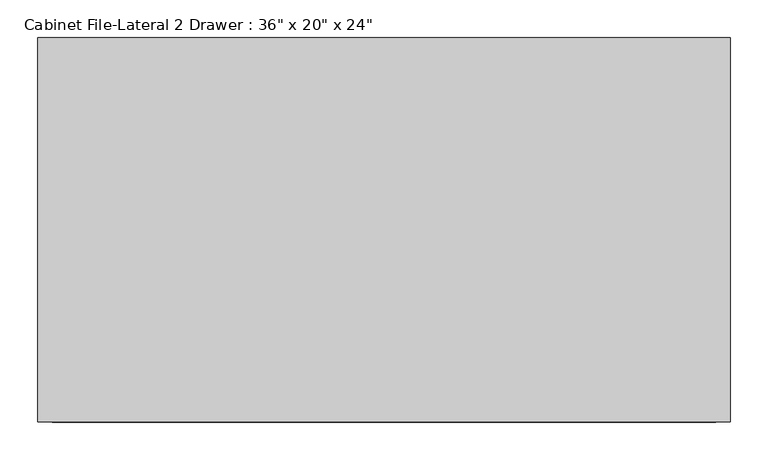
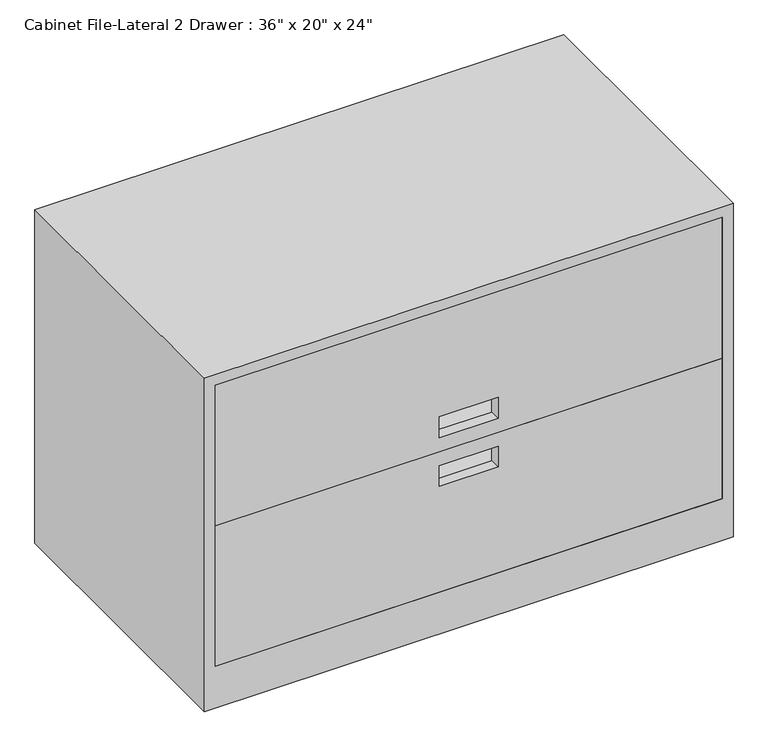
"""IFC4 building model written with IfcOpenShell, lengths in millimetres: furniture geometry."""

from ifc_helpers import new_model, si_unit, frame, origin, place, context, project, spatial, polyline, outline, extrude, faceted_brep, source, transform, mapped, element, save


def furniture_6b884072(model_context):
    return source(origin(), model_context, "Body", "SolidModel", [
        faceted_brep([(277.1774861, -680.3183761, 609.6), (-637.2225139, -680.3183761, 609.6), (-637.2225139, -1188.3183761, 609.6), (277.1774861, -1188.3183761, 609.6), (277.1774861, -680.3183761, 0.0), (277.1774861, -1188.3183761, 0.0), (-637.2225139, -1188.3183761, 0.0), (-637.2225139, -680.3183761, 0.0), (258.1274861, -1188.3183761, 76.2), (-618.1725139, -1188.3183761, 76.2), (-618.1725139, -1188.3183761, 590.55), (258.1274861, -1188.3183761, 590.55), (-618.1725139, -699.3683761, 76.2), (258.1274861, -699.3683761, 76.2), (258.1274861, -699.3683761, 590.55), (-618.1725139, -699.3683761, 590.55)], [[[0, 1, 2, 3]], [[4, 5, 6, 7]], [[1, 0, 4, 7]], [[2, 1, 7, 6]], [[3, 2, 6, 5], [8, 9, 10, 11]], [[0, 3, 5, 4]], [[12, 13, 14, 15]], [[13, 12, 9, 8]], [[14, 13, 8, 11]], [[15, 14, 11, 10]], [[12, 15, 10, 9]]]),
        extrude(outline(polyline([(333.375, -618.1725139), (333.375, 258.1274861), (590.55, 258.1274861), (590.55, -618.1725139), (333.375, -618.1725139)]), holes=[polyline([(396.875, -230.8225139), (396.875, -129.2225139), (358.775, -129.2225139), (358.775, -230.8225139), (396.875, -230.8225139)])]), frame((0.0, -1188.3183761, 0.0), z_axis=(0.0, 1.0, 0.0), x_axis=(0.0, 0.0, 1.0)), (0.0, 0.0, 1.0), 19.05),
        extrude(outline(polyline([(76.2, -618.1725139), (76.2, 258.1274861), (333.375, 258.1274861), (333.375, -618.1725139), (76.2, -618.1725139)]), holes=[polyline([(307.975, -230.8225139), (307.975, -129.2225139), (269.875, -129.2225139), (269.875, -230.8225139), (307.975, -230.8225139)])]), frame((0.0, -1188.3183761, 0.0), z_axis=(0.0, 1.0, 0.0), x_axis=(0.0, 0.0, 1.0)), (0.0, 0.0, 1.0), 19.05),
    ])


if __name__ == "__main__":
    model = new_model("IFC4")
    model_context = context("Model", 3, world=origin())
    ifc_project = project(units=[si_unit("LENGTHUNIT", "METRE", prefix="MILLI")], contexts=[model_context])
    site = spatial("IfcSite", under=ifc_project)
    building = spatial("IfcBuilding", under=site)
    placement = place(None, origin())
    furniture_shape = furniture_6b884072(model_context)
    element("IfcFurniture", 1, ObjectType="Cabinet File-Lateral 2 Drawer : 36\" x 20\" x 24\"", at=placement, inside=building, context=model_context, shape_type="MappedRepresentation", body=[
        mapped(furniture_shape, transform((0.0, 0.0, 0.0), x_axis=(1.0, 0.0, 0.0), y_axis=(0.0, 1.0, 0.0), z_axis=(0.0, 0.0, 1.0))),
    ])
    save(model, "model.ifc")

# Revit data of these elements
# Type "Cabinet File-Lateral 2 Drawer : 36\" x 20\" x 24\""
#   Assembly Code = "E2020200"
#   Depth = 1' - 8"
#   Height = 2' - 0"
#   Width = 3' - 0"
#   Material = Metal - Steel
#   Default Elevation = 0
# Element 1 (IfcFurniture, "Cabinet File-Lateral 2 Drawer : 36\" x 20\" x 24\"")
#   Materials on its faces: "Metal - Steel"
# Materials
#   "Metal - Steel": colour RGB 209 209 209, transparency 0
